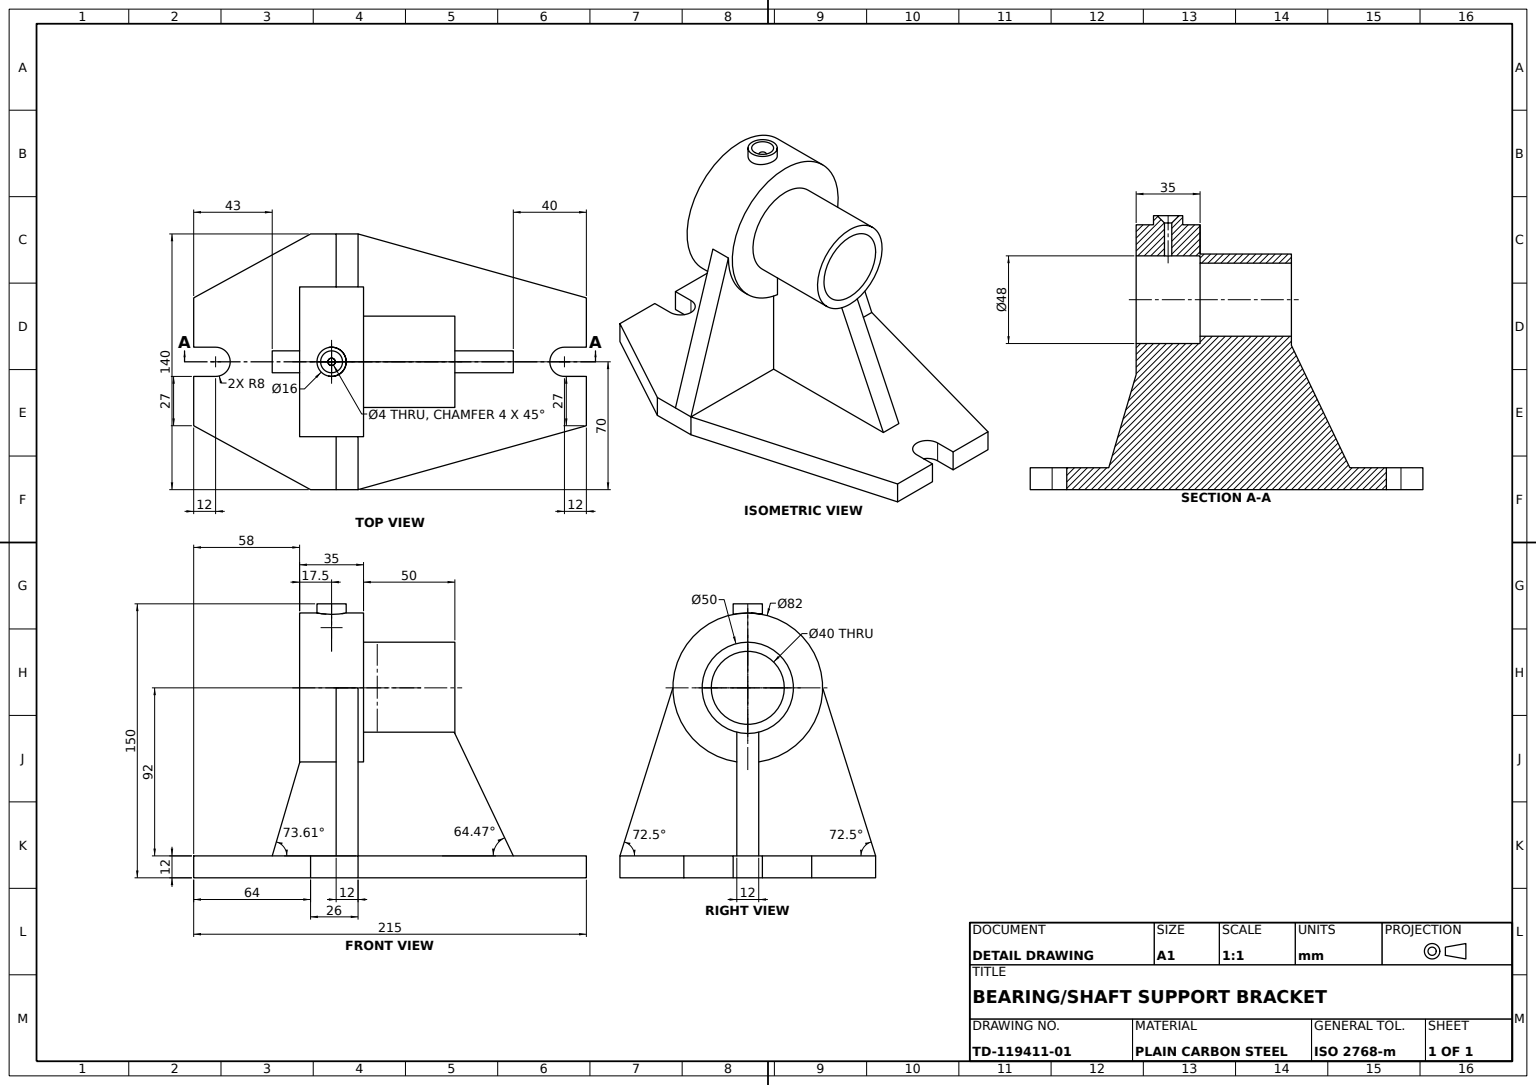
SolidWorks part; units mm, degrees
material "Plain Carbon Steel"
ref_plane "Front Plane" through (0, 0, 0) normal (0, 0, 1) x (1, 0, 0)
ref_plane "Top Plane" through (0, 0, 0) normal (0, 1, 0) x (1, 0, 0)
ref_plane "Right Plane" through (0, 0, 0) normal (1, 0, 0) x (0, 0, -1)
sketch "Base Plate Sketch" plane through (0, 0, 0) normal (0, 1, 0) x (1, 0, 0)
  line L0 (-90, -35) -> (-90, -8)
  line L1 (-90, 35) -> (-26, 70)
  line L2 (-26, 70) -> (0, 70)
  line L3 (0, 70) -> (125, 35)
  line L4 (125, 35) -> (125, 8)
  line L5 (125, -35) -> (0, -70)
  line L6 (0, -70) -> (-26, -70)
  line L7 (-26, -70) -> (-90, -35)
  line L8 (0, 0) -> (33.1111, 0) construction
  line L9 (-78, 8) -> (-90, 8)
  line L11 (-90, -8) -> (-78, -8)
  line L12 (-90, 8) -> (-90, 35)
  line L13 (113, 8) -> (125, 8)
  line L14 (113, -8) -> (125, -8)
  line L15 (125, -8) -> (125, -35)
  arc A0 (-78, -8) -> (-78, 8) centre (-78, 0) ccw
  arc A1 (113, 8) -> (113, -8) centre (113, 0) ccw
  dimension "D1" = 26
  dimension "D2" = 12
  dimension "D3" = 27
  dimension "D4" = 16
  dimension "D5" = 140
  dimension "D6" = 125
  dimension "D7" = 12
  dimension "D8" = 27
  dimension "D9" = 16
  dimension "D10" = 64
extrude "Base Plate" add sketch "Base Plate Sketch" along normal blind 12
sketch "Bearing Boss Profile" plane through (0, 0, 0) normal (0, 0, 1) x (1, 0, 0)
  line L1 (53, 104) -> (-32, 104)
  line L2 (-32, 104) -> (-32, 63)
  line L3 (-32, 63) -> (3, 63)
  line L4 (3, 63) -> (3, 79)
  line L5 (3, 79) -> (53, 79)
  line L6 (53, 79) -> (53, 104)
  line L7 (0, 12) -> (125, 12) construction
  dimension "D1" = 92
  dimension "D2" = 25
  dimension "D3" = 41
  dimension "D4" = 50
  dimension "D5" = 35
  dimension "D6" = 3
revolve "Bearing Boss" add sketch "Bearing Boss Profile" angle 360 about L1
sketch "Stepped Bore Profile" plane through (0, 0, 0) normal (0, 0, 1) x (1, 0, 0)
  line L0 (-32, 128) -> (3, 128)
  line L1 (-32, 145) -> (-32, 63) construction
  line L2 (3, 63) -> (3, 145) construction
  line L3 (-32, 128) -> (-32, 104)
  line L4 (-32, 104) -> (53, 104)
  line L5 (53, 79) -> (53, 129) construction
  line L6 (53, 104) -> (53, 124)
  line L7 (53, 124) -> (3, 124)
  line L8 (3, 79) -> (3, 129) construction
  line L9 (3, 124) -> (3, 128)
  dimension "D1" = 24
  dimension "D2" = 20
revolve "Stepped Bore" cut sketch "Stepped Bore Profile" angle 360 about L4
sketch "Support Web Sketch" plane through (0, 0, 0) normal (1, 0, 0) x (0, 0, -1)
  line L0 (-70, 12) -> (-41, 104)
  line L1 (-35, 12) -> (-8, 12) construction
  line L2 (70, 12) -> (41, 104)
  line L3 (35, 12) -> (70, 12) construction
  line L4 (8, 12) -> (35, 12) construction
  line L5 (8, 12) -> (-8, 12) construction
  line L6 (-70, 12) -> (-35, 12) construction
  line L7 (35, 12) -> (70, 12)
  line L8 (8, 12) -> (35, 12)
  line L9 (8, 12) -> (-8, 12)
  line L10 (-70, 12) -> (-35, 12)
  line L11 (-35, 12) -> (-8, 12)
  circle A0 centre (0, 104) radius 41 construction
  arc A1 (-41, 104) -> (41, 104) centre (0, 104) ccw
  dimension "D1" = 92
extrude "Support Web" add sketch "Support Web Sketch" against normal blind 12
sketch "Web Gusset Rib Sketch" plane through (0, 0, 0) normal (0, 0, 1) x (1, 0, 0)
  line L0 (-32, 63) -> (-47, 12)
  line L1 (-90, 12) -> (-26, 12) construction
  line L3 (-12, 104) -> (-12, 12) construction
  dimension "D1" = 35
rib "Web Gusset Rib" sketch "Web Gusset Rib Sketch" sketch "Web Gusset Rib Sketch" thickness 12 extrusion direction parallel to sketch draft on no parameters "D1"=12
sketch "Side Gusset Rib Sketch" plane through (0, 0, 0) normal (0, 0, 1) x (1, 0, 0)
  line L0 (53, 79) -> (85, 12)
  line L1 (0, 12) -> (125, 12) construction
  line L2 (125, 12) -> (125, 0) construction
  dimension "D1" = 40
rib "Side Gusset Rib" sketch "Side Gusset Rib Sketch" sketch "Side Gusset Rib Sketch" thickness 12 extrusion direction parallel to sketch draft on no parameters "D1"=12
ref_plane "Grease Boss Plane" through (0, 150, 0) normal (0, 1, 0) x (1, 0, 0)
sketch "Grease Boss Sketch" plane through (0, 150, 0) normal (0, 1, 0) x (1, 0, 0)
  line L1 (3, -41) -> (3, 41) construction
  circle A0 centre (-14.5, 0) radius 8
  dimension "D1" = 16
  dimension "D2" = 17.5
extrude "Grease Boss Ø16" add sketch "Grease Boss Sketch" against normal up to surface (5.7881 mm away)
sketch "Lube Hole Sketch" plane through (0, 150, 0) normal (0, 1, 0) x (1, 0, 0)
  circle A0 centre (-14.5, 0) radius 2
  circle A1 centre (-14.5, 0) radius 8 construction
  dimension "D1" = 4
extrude "Lube Hole" cut sketch "Lube Hole Sketch" against normal blind 35
chamfer "Grease Boss Chamfer 4x45°" distance 4 angle 45 1 edges at (-14.5, 150, 2)
